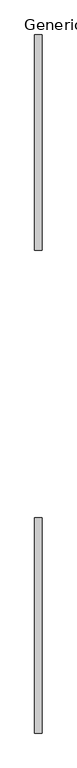
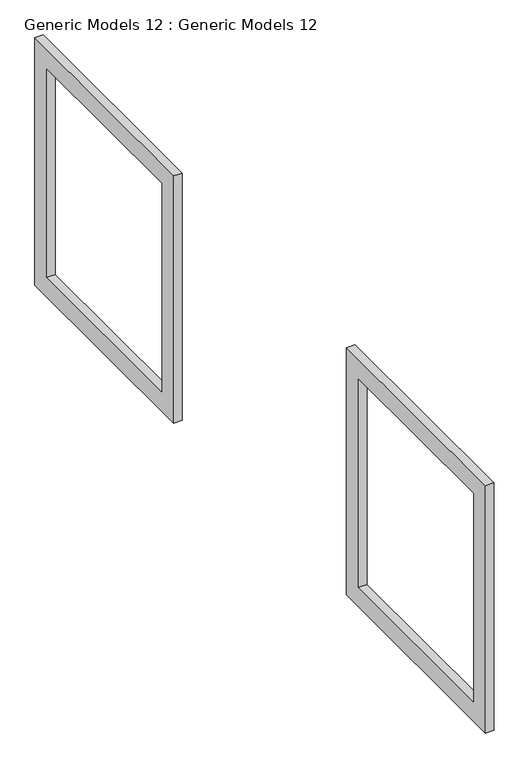
"""IFC4 building model written with IfcOpenShell, lengths in millimetres: proxy geometry, Generic Models 12 : Generic Models 12."""

from ifc_helpers import new_model, si_unit, frame, origin, place, context, project, spatial, polyline, outline, extrude, source, transform, mapped, element, save


def generic_models_12_generic_models_12_bd71d687(model_context):
    return source(origin(), model_context, "Body", "SweptSolid", [
        extrude(outline(polyline([(744.7157342, 2692.4), (744.7157342, 1092.2), (-728.4842658, 1092.2), (-728.4842658, 2692.4), (744.7157342, 2692.4)]), holes=[polyline([(617.7157342, 2565.4), (-601.4842658, 2565.4), (-601.4842658, 1219.2), (617.7157342, 1219.2), (617.7157342, 2565.4)])]), frame((-2406.7607439, 0.0, 0.0), z_axis=(1.0, 0.0, 0.0), x_axis=(0.0, 1.0, 0.0)), (0.0, 0.0, 1.0), 50.8),
        extrude(outline(polyline([(4051.566494, 2692.4), (4051.566494, 1092.2), (2578.366494, 1092.2), (2578.366494, 2692.4), (4051.566494, 2692.4)]), holes=[polyline([(3924.566494, 2565.4), (2705.366494, 2565.4), (2705.366494, 1219.2), (3924.566494, 1219.2), (3924.566494, 2565.4)])]), frame((-2406.7607439, 0.0, 0.0), z_axis=(1.0, 0.0, 0.0), x_axis=(0.0, 1.0, 0.0)), (0.0, 0.0, 1.0), 50.8),
    ])


if __name__ == "__main__":
    model = new_model("IFC4")
    model_context = context("Model", 3, world=origin())
    ifc_project = project(units=[si_unit("LENGTHUNIT", "METRE", prefix="MILLI")], contexts=[model_context])
    site = spatial("IfcSite", under=ifc_project)
    building = spatial("IfcBuilding", under=site)
    placement = place(None, origin())
    generic_models_12_generic_models_12_shape = generic_models_12_generic_models_12_bd71d687(model_context)
    element("IfcBuildingElementProxy", 1, Name="Generic Models 12 : Generic Models 12", ObjectType="Generic Models 12 : Generic Models 12", at=placement, inside=building, context=model_context, shape_type="MappedRepresentation", body=[
        mapped(generic_models_12_generic_models_12_shape, transform((0.0, 0.0, 0.0), x_axis=(1.0, 0.0, 0.0), y_axis=(0.0, 1.0, 0.0), z_axis=(0.0, 0.0, 1.0))),
    ])
    save(model, "model.ifc")

# Revit data of these elements
# Element 1 (IfcBuildingElementProxy, "Generic Models 12 : Generic Models 12")
#   Materials on its faces: "BLACK"
# Materials
#   "BLACK": class "Generic", colour RGB 120 120 120, transparency 0, Cost = 0
